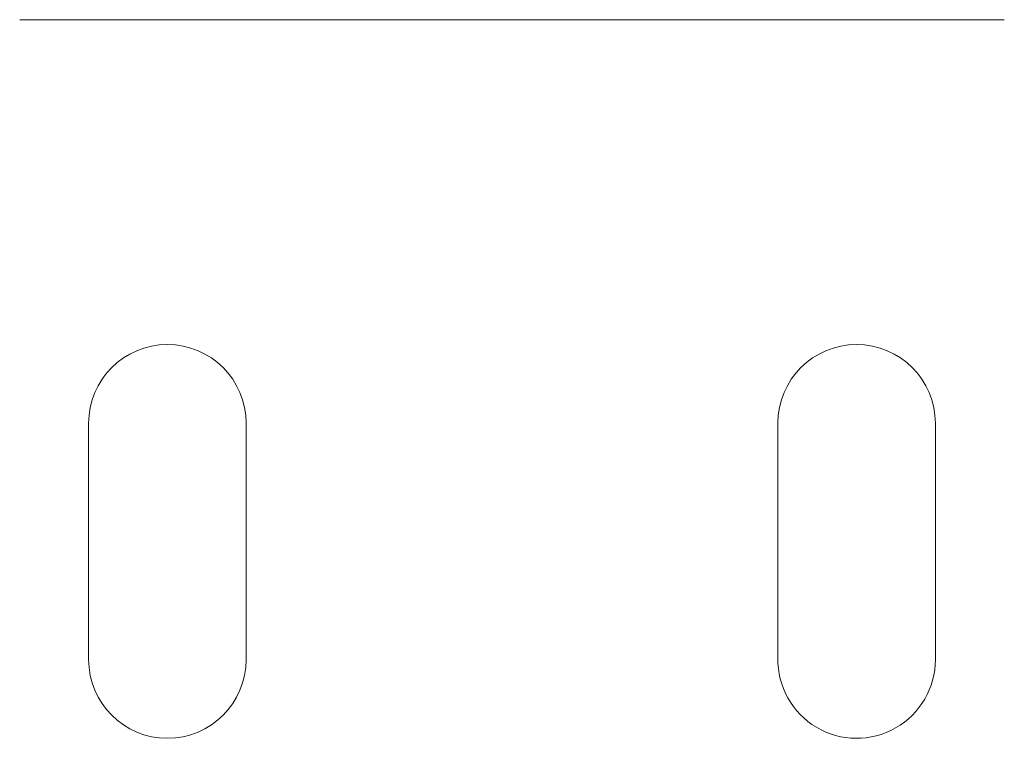
# Model space of a CAD drawing. Units: millimetres. Extents: x 464.6 to 564.6, y -73 to 0.
import ezdxf

# ---------------------------------------------------------------- set-up
doc = ezdxf.new("R2010")
doc.units = ezdxf.units.MM
doc.layers.add('M-CONS', color=8, linetype='Continuous', lineweight=18)

msp = doc.modelspace()

# ---------------------------------------------------------------- linework, layer by layer
at = {"layer": 'M-CONS', "extrusion": (0, -1, 0)}
for p, q in [((464.59, 0, 133.52), (464.59, 0, 153.52)), ((464.59, 0, 153.52), (564.59, 0, 153.52)), ((564.59, 0, 133.52), (464.59, 0, 133.52)), ((464.59, 0, 193.52), (469.59, 0, 193.52)), ((484.59, 0, 283.52), (484.59, 0, 208.52)), ((502.59, 0, 283.52), (502.59, 0, 213.52)), ((514.59, 0, 153.52), (564.59, 0, 153.52)), ((526.59, 0, 283.52), (526.59, 0, 213.52)), ((544.59, 0, 283.52), (544.59, 0, 214.34)), ((544.59, 0, 214.34), (544.59, 0, 208.52)), ((564.59, 0, 193.52), (559.59, 0, 193.52)), ((564.59, 0, 153.52), (564.59, 0, 133.52)), ((564.59, 0, 153.52), (564.59, 0, 193.52))]:
    msp.add_line(p, q, dxfattribs=at)
at = {"layer": 'M-CONS', "extrusion": (-1, 0, 0)}
msp.add_line((464.59, 0, 153.52), (464.59, 0, 193.52), dxfattribs=at)
at = {"layer": 'M-CONS'}
for p, q in [((471.59, -41, 153.52), (471.59, -65, 153.52)), ((487.59, -65, 153.52), (487.59, -41, 153.52)), ((541.59, -41, 153.52), (541.59, -65, 153.52)), ((557.59, -41, 153.52), (557.59, -65, 153.52)), ((557.59, -65.14, 153.52), (557.59, -65.14, 153.52))]:
    msp.add_line(p, q, dxfattribs=at)
at = {"layer": 'M-CONS', "extrusion": (0, -1, 0)}
for centre in [(489.59, 173.52), (539.59, 173.52)]:
    msp.add_circle(centre, 12, dxfattribs=at)
for centre, radius, start, end in [((469.59, 208.52), 15, 270, 0), ((514.59, 283.52), 30, 0, 180), ((514.59, 283.52), 12, 0, 180), ((514.59, 213.52), 12, 180, 0), ((559.59, 208.52), 15, 180, 270)]:
    msp.add_arc(centre, radius, start, end, dxfattribs=at)
at = {"layer": 'M-CONS'}
for centre, start, end in [((479.59, -41, 153.52), 0, 180), ((549.59, -41, 153.52), 0, 180), ((549.59, -65, 153.52), 178.9852, 0), ((479.59, -65, 153.52), 180, 0)]:
    msp.add_arc(centre, 8, start, end, dxfattribs=at)

doc.saveas('drawing.dxf')
